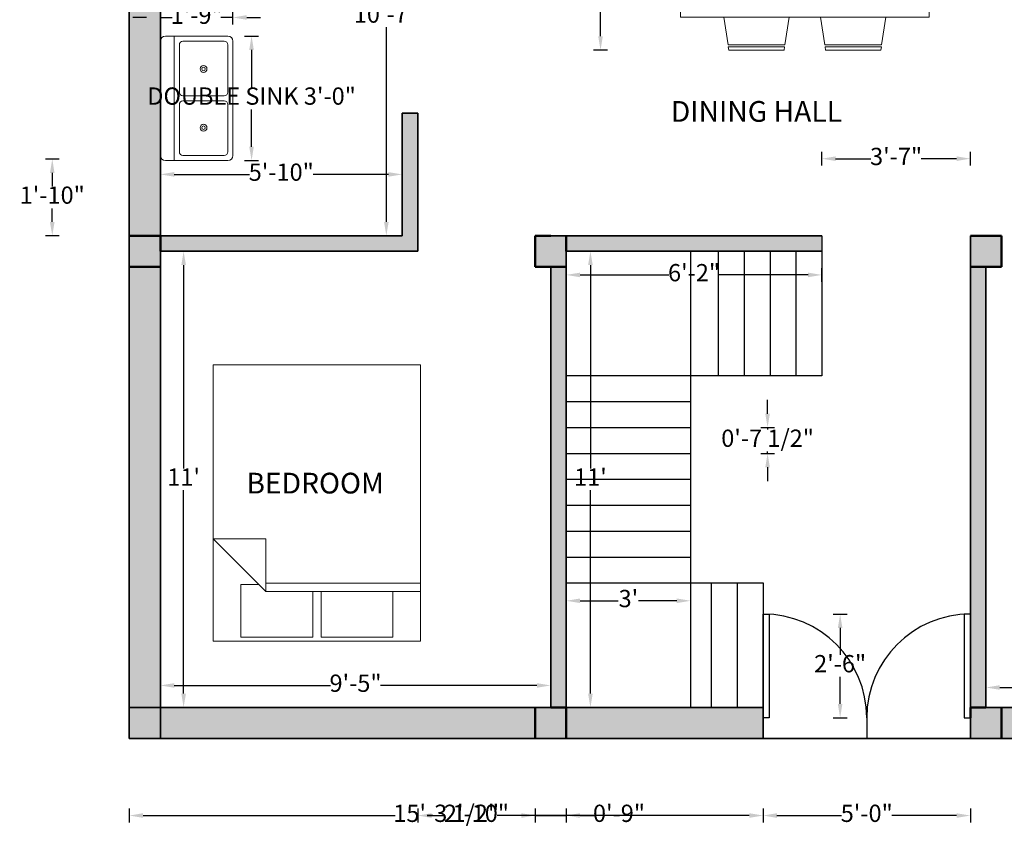
# Model space of a CAD drawing. Units: inches. Extents: x 2244 to 2676, y 593 to 1067.
# Tile 1 of 4: x 2244 to 2530, y 593 to 831. Entities that reach past the tile are written whole.
import ezdxf

# ---------------------------------------------------------------- set-up
doc = ezdxf.new("R2010")
doc.units = ezdxf.units.IN
for name, color, linetype, lineweight in [('A-ANNO-DIMS', 2, 'Continuous', 18), ('A-AREA-IDEN', 7, 'Continuous', 25), ('A-COLS', 7, 'Continuous', 50), ('A-COLS-PATT', 1, 'Continuous', 13), ('A-DOOR', 4, 'Continuous', 25), ('A-FLOR-FIXT', 9, 'Continuous', 18), ('A-FLOR-STRS', 7, 'Continuous', 25), ('A-FURN', 8, 'Continuous', 18), ('A-WALL', 7, 'Continuous', 35)]:
    doc.layers.add(name, color=color, linetype=linetype, lineweight=lineweight)
doc.layers.add('A-WALL-PATT', color=159, linetype='Continuous', lineweight=13, true_color=0x22346e)
doc.styles.get("Standard").update_dxf_attribs({"font": 'arial.ttf'})
doc.dimstyles.new('ISO-25', dxfattribs={"dimtxt": 5, "dimasz": 4, "dimexe": 2, "dimexo": 2, "dimtad": 0, "dimtih": 1, "dimtoh": 1, "dimlunit": 3, "dimtxsty": 'Standard', "dimcen": 2.5, "dimadec": 0, "dimazin": 0, "dimtfac": 1, "dimtmove": 0, "dimatfit": 3, "dimfxl": 2, "dimfxlon": 1, "dimarcsym": 0})

# ---------------------------------------------------------------- blocks, each defined once
blk = doc.blocks.new('*U2')
for p, q in [((0, 0), (0, -6)), ((30, 0), (30, -6))]:
    blk.add_line(p, q)
blk.add_lwpolyline([(0, 0), (0, 30), (1.75, 30), (1.75, 0)], close=True)
blk.add_arc((0, 0), 30, 0, 90)
blk = doc.blocks.new('*U3')
for p, q in [((-30, 0), (-30, -6)), ((0, 0), (0, -6))]:
    blk.add_line(p, q)
blk.add_lwpolyline([(0, 0), (0, 30), (-1.75, 30), (-1.75, 0)], close=True)
blk.add_arc((0, 0), 30, 90, 180)
blk = doc.blocks.new('*D10')
at = {"layer": 'A-ANNO-DIMS', "color": 0, "lineweight": -2, "transparency": 16777216}
for p, q in [((2285.2, 784.43), (2285.2, 788.17)), ((2355.2, 784.43), (2355.2, 788.17)), ((2289.2, 786.17), (2310.98, 786.17)), ((2351.2, 786.17), (2329.41, 786.17))]:
    blk.add_line(p, q, dxfattribs=at)
at = {"layer": 'A-ANNO-DIMS', "color": 0, "transparency": 16777216}
for points in [[(2289.2, 786.84), (2289.2, 785.5), (2285.2, 786.17)], [(2351.2, 786.84), (2351.2, 785.5), (2355.2, 786.17)]]:
    blk.add_solid(points, dxfattribs=at)
at = {"layer": 'Defpoints', "color": 0, "transparency": 16777216}
for p in [(2355.2, 786.17), (2285.2, 782.43), (2355.2, 782.43)]:
    blk.add_point(p, dxfattribs=at)
at = {"layer": 'A-ANNO-DIMS', "color": 0, "transparency": 16777216, "insert": (2320.2, 786.17), "char_height": 5, "attachment_point": 5}
blk.add_mtext('5\'-10"', dxfattribs=at)
blk = doc.blocks.new('*D15')
at = {"layer": 'A-ANNO-DIMS', "color": 0, "lineweight": -2, "transparency": 16777216}
for p, q in [((2524.2, 639.68), (2524.2, 635.68)), ((2637.2, 639.68), (2637.2, 635.68)), ((2528.2, 637.68), (2573.43, 637.68)), ((2633.2, 637.68), (2587.97, 637.68))]:
    blk.add_line(p, q, dxfattribs=at)
at = {"layer": 'A-ANNO-DIMS', "color": 0, "transparency": 16777216}
for points in [[(2528.2, 638.34), (2528.2, 637.01), (2524.2, 637.68)], [(2633.2, 638.34), (2633.2, 637.01), (2637.2, 637.68)]]:
    blk.add_solid(points, dxfattribs=at)
at = {"layer": 'Defpoints', "color": 0, "transparency": 16777216}
for p in [(2524.2, 645.95), (2637.2, 645.95), (2637.2, 637.68)]:
    blk.add_point(p, dxfattribs=at)
at = {"layer": 'A-ANNO-DIMS', "color": 0, "transparency": 16777216, "insert": (2580.7, 637.68), "char_height": 5, "attachment_point": 5}
blk.add_mtext('9\'-5"', dxfattribs=at)
blk = doc.blocks.new('*D16')
at = {"layer": 'A-ANNO-DIMS', "color": 0, "lineweight": -2, "transparency": 16777216}
for p, q in [((2402.7, 755.08), (2402.7, 759.08)), ((2476.7, 755.08), (2476.7, 759.08)), ((2406.7, 757.08), (2432.41, 757.08)), ((2472.7, 757.08), (2446.98, 757.08))]:
    blk.add_line(p, q, dxfattribs=at)
at = {"layer": 'A-ANNO-DIMS', "color": 0, "transparency": 16777216}
for points in [[(2406.7, 757.74), (2406.7, 756.41), (2402.7, 757.08)], [(2472.7, 757.74), (2472.7, 756.41), (2476.7, 757.08)]]:
    blk.add_solid(points, dxfattribs=at)
at = {"layer": 'Defpoints', "color": 0, "transparency": 16777216}
for p in [(2476.7, 757.08), (2402.7, 743.42), (2476.7, 743.42)]:
    blk.add_point(p, dxfattribs=at)
at = {"layer": 'A-ANNO-DIMS', "color": 0, "transparency": 16777216, "insert": (2439.7, 757.08), "char_height": 5, "attachment_point": 5}
blk.add_mtext('6\'-2"', dxfattribs=at)
blk = doc.blocks.new('*D17')
at = {"layer": 'A-ANNO-DIMS', "color": 0, "lineweight": -2, "transparency": 16777216}
for p, q in [((2411.7, 763.92), (2407.7, 763.92)), ((2409.7, 759.92), (2409.7, 701.06)), ((2409.7, 635.92), (2409.7, 694.79)), ((2411.7, 631.92), (2407.7, 631.92))]:
    blk.add_line(p, q, dxfattribs=at)
at = {"layer": 'A-ANNO-DIMS', "color": 0, "transparency": 16777216}
for points in [[(2409.03, 759.92), (2410.37, 759.92), (2409.7, 763.92)], [(2409.03, 635.92), (2410.37, 635.92), (2409.7, 631.92)]]:
    blk.add_solid(points, dxfattribs=at)
at = {"layer": 'Defpoints', "color": 0, "transparency": 16777216}
for p in [(2415.93, 763.92), (2409.7, 631.92), (2415.93, 631.92)]:
    blk.add_point(p, dxfattribs=at)
at = {"layer": 'A-ANNO-DIMS', "color": 0, "transparency": 16777216, "insert": (2409.7, 697.92), "char_height": 5, "attachment_point": 5}
blk.add_mtext("11'", dxfattribs=at)
blk = doc.blocks.new('*D18')
at = {"layer": 'A-ANNO-DIMS', "color": 0, "lineweight": -2, "transparency": 16777216}
for p, q in [((2402.7, 664.77), (2402.7, 660.77)), ((2438.7, 664.77), (2438.7, 660.77)), ((2406.7, 662.77), (2417.77, 662.77)), ((2434.7, 662.77), (2423.62, 662.77))]:
    blk.add_line(p, q, dxfattribs=at)
at = {"layer": 'A-ANNO-DIMS', "color": 0, "transparency": 16777216}
for points in [[(2406.7, 663.44), (2406.7, 662.11), (2402.7, 662.77)], [(2434.7, 663.44), (2434.7, 662.11), (2438.7, 662.77)]]:
    blk.add_solid(points, dxfattribs=at)
at = {"layer": 'Defpoints', "color": 0, "transparency": 16777216}
for p in [(2402.7, 667.92), (2438.7, 667.92), (2438.7, 662.77)]:
    blk.add_point(p, dxfattribs=at)
at = {"layer": 'A-ANNO-DIMS', "color": 0, "transparency": 16777216, "insert": (2420.7, 662.77), "char_height": 5, "attachment_point": 5}
blk.add_mtext("3'", dxfattribs=at)
blk = doc.blocks.new('*D19')
at = {"layer": 'A-ANNO-DIMS', "color": 0, "lineweight": -2, "transparency": 16777216}
for p, q in [((2291.93, 763.92), (2289.93, 763.92)), ((2291.93, 759.92), (2291.93, 701.06)), ((2291.93, 635.92), (2291.93, 694.79)), ((2291.93, 631.92), (2289.93, 631.92))]:
    blk.add_line(p, q, dxfattribs=at)
at = {"layer": 'A-ANNO-DIMS', "color": 0, "transparency": 16777216}
for points in [[(2291.27, 759.92), (2292.6, 759.92), (2291.93, 763.92)], [(2291.27, 635.92), (2292.6, 635.92), (2291.93, 631.92)]]:
    blk.add_solid(points, dxfattribs=at)
at = {"layer": 'Defpoints', "color": 0, "transparency": 16777216}
for p in [(2292.44, 763.92), (2291.93, 631.92), (2292.44, 631.92)]:
    blk.add_point(p, dxfattribs=at)
at = {"layer": 'A-ANNO-DIMS', "color": 0, "transparency": 16777216, "insert": (2291.93, 697.92), "char_height": 5, "attachment_point": 5}
blk.add_mtext("11'", dxfattribs=at)
blk = doc.blocks.new('*D20')
at = {"layer": 'A-ANNO-DIMS', "color": 0, "lineweight": -2, "transparency": 16777216}
for p, q in [((2285.2, 640.27), (2285.2, 636.27)), ((2398.2, 640.27), (2398.2, 636.27)), ((2289.2, 638.27), (2334.43, 638.27)), ((2394.2, 638.27), (2348.97, 638.27))]:
    blk.add_line(p, q, dxfattribs=at)
at = {"layer": 'A-ANNO-DIMS', "color": 0, "transparency": 16777216}
for points in [[(2289.2, 638.93), (2289.2, 637.6), (2285.2, 638.27)], [(2394.2, 638.93), (2394.2, 637.6), (2398.2, 638.27)]]:
    blk.add_solid(points, dxfattribs=at)
at = {"layer": 'Defpoints', "color": 0, "transparency": 16777216}
for p in [(2285.2, 662.54), (2398.2, 662.54), (2398.2, 638.27)]:
    blk.add_point(p, dxfattribs=at)
at = {"layer": 'A-ANNO-DIMS', "color": 0, "transparency": 16777216, "insert": (2341.7, 638.27), "char_height": 5, "attachment_point": 5}
blk.add_mtext('9\'-5"', dxfattribs=at)
blk = doc.blocks.new('Bed - Queen')
for p, q in [((0, -80.00003), (0, 0)), ((0, 0), (59.99999, 0)), ((59.99999, 0), (59.99999, -80.00003)), ((7.99999, -1.2), (28.79998, -1.2)), ((7.99999, -14.4), (7.99999, -1.2)), ((28.79998, -1.2), (28.79998, -14.4)), ((31.19999, -1.2), (51.99999, -1.2)), ((31.19999, -14.4), (31.19999, -1.2)), ((51.99999, -1.2), (51.99999, -16.4)), ((0, -14.4), (44.8, -14.4)), ((44.8, -16.8), (0, -16.8)), ((59.99999, -29.6), (44.8, -14.4)), ((44.8, -14.4), (44.8, -29.6)), ((51.99999, -16.4), (46.79936, -16.4)), ((44.8, -29.6), (59.99999, -29.6)), ((59.99999, -80.00003), (0, -80.00003))]:
    blk.add_line(p, q)
blk = doc.blocks.new('Dining Set - 36 x 72 in.')
for p, q in [((-22.2343, 26.00059), (-23.4847, 17.99762)), ((-22.2304, 26), (-5.7608, 26)), ((-22, 27.5), (-22.1562, 26.50042)), ((-5.8416, 26.5), (-22.1534, 26.5)), ((-22, 27.5), (-6, 27.5)), ((-5.8437, 26.49966), (-6, 27.5)), ((-4.5152, 17.99762), (-5.7655, 25.99926)), ((5.7657, 26.00059), (4.5153, 17.99762)), ((5.7696, 26), (22.2392, 26)), ((6, 27.5), (5.8438, 26.50042)), ((22.1584, 26.5), (5.8466, 26.5)), ((6, 27.5), (22, 27.5)), ((22.1563, 26.49966), (22, 27.5)), ((23.4848, 17.99762), (22.2345, 25.99926)), ((36, 18), (-36, 18)), ((-36, 18), (-36, -18)), ((36, -18), (36, 18)), ((-44.0006, 8.23428), (-35.9976, 9.48474)), ((44.0006, 8.23428), (35.9976, 9.48474)), ((-45.5, 8), (-44.5004, 8.15617)), ((-45.5, 8), (-45.5, -8)), ((-44.5, -8.15843), (-44.5, 8.15338)), ((-44, 8.23041), (-44, -8.23915)), ((44, 8.23041), (44, -8.23915)), ((44.5, -8.15843), (44.5, 8.15338)), ((45.5, 8), (44.5005, 8.15617)), ((45.5, 8), (45.5, -8)), ((-44.4997, -8.15631), (-45.5, -8)), ((-35.9976, -9.48476), (-43.9993, -8.2345)), ((35.9976, -9.48476), (43.9993, -8.2345)), ((44.4997, -8.15631), (45.5, -8)), ((-36, -18), (36, -18)), ((-22.2343, -26.0006), (-23.4847, -17.99762)), ((-4.5152, -17.99762), (-5.7655, -25.99928)), ((5.7657, -26.0006), (4.5153, -17.99762)), ((23.4848, -17.99762), (22.2345, -25.99928)), ((-22.2304, -26), (-5.7608, -26)), ((-22, -27.5), (-22.1562, -26.50044)), ((-5.8416, -26.5), (-22.1534, -26.5)), ((-22, -27.5), (-6, -27.5)), ((-5.8437, -26.49967), (-6, -27.5)), ((5.7696, -26), (22.2392, -26)), ((6, -27.5), (5.8438, -26.50044)), ((22.1584, -26.5), (5.8466, -26.5)), ((6, -27.5), (22, -27.5)), ((22.1563, -26.49967), (22, -27.5))]:
    blk.add_line(p, q)
for points in [[(-36, 15), (-31.1772, 14.97754), (-26.8079, 14.91406), (-22.8538, 14.81543), (-19.276, 14.6875), (-16.0362, 14.53613), (-13.0957, 14.36718), (-10.4159, 14.18652), (-7.9583, 14), (-5.6904, 13.81315), (-3.6035, 13.63021), (-1.6954, 13.45508), (0.0365, 13.29166), (1.5945, 13.14388), (2.9811, 13.01562), (4.1988, 12.9108), (5.25, 12.83333), (6.1393, 12.78613), (6.8802, 12.76823), (7.4883, 12.77767), (7.9792, 12.8125), (8.3685, 12.87077), (8.6719, 12.95052), (8.9049, 13.0498), (9.0833, 13.16666), (9.2205, 13.29899), (9.3216, 13.44401), (9.3895, 13.59879), (9.4271, 13.76041), (9.4373, 13.92594), (9.4232, 14.09245), (9.3875, 14.257), (9.3333, 14.41666), (9.2638, 14.56917), (9.1836, 14.71484), (9.0975, 14.85465), (9.0104, 14.98958), (8.9272, 15.1206), (8.8529, 15.2487), (8.7922, 15.37483), (8.75, 15.5), (8.7305, 15.62467), (8.7344, 15.74739), (8.7617, 15.86621), (8.8125, 15.97916), (8.8867, 16.08431), (8.9844, 16.17968), (9.1055, 16.26334), (9.25, 16.33333), (9.4189, 16.38802), (9.6172, 16.42708), (9.8506, 16.45052), (10.125, 16.45833), (10.4463, 16.45052), (10.8203, 16.42708), (11.2529, 16.38802), (11.75, 16.33333), (12.3184, 16.26318), (12.9694, 16.17838), (13.7151, 16.07991), (14.5677, 15.96875), (15.5395, 15.84586), (16.6426, 15.71224), (17.8893, 15.56884), (19.2917, 15.41666), (20.859, 15.25667), (22.5879, 15.08984), (24.4721, 14.91715), (26.5052, 14.73958), (28.6809, 14.5581), (30.9929, 14.3737), (33.4347, 14.18733), (36, 14)], [(-36, 10), (-28.9766, 10.14274), (-23.1725, 10.20442), (-18.4241, 10.19775), (-14.5677, 10.13541), (-11.4399, 10.03011), (-8.877, 9.89453), (-6.7154, 9.74137), (-4.7917, 9.58333), (-2.9698, 9.43082), (-1.2246, 9.28515), (0.4415, 9.14534), (2.026, 9.01041), (3.5266, 8.87939), (4.9408, 8.7513), (6.266, 8.62516), (7.5, 8.5), (8.6411, 8.37549), (9.6914, 8.2539), (10.6538, 8.13818), (11.5312, 8.03125), (12.3267, 7.93603), (13.043, 7.85547), (13.6831, 7.79248), (14.25, 7.75), (14.7471, 7.7303), (15.1797, 7.73307), (15.5537, 7.75732), (15.875, 7.80208), (16.1494, 7.86637), (16.3828, 7.94922), (16.5811, 8.04964), (16.75, 8.16666), (16.8944, 8.29915), (17.0143, 8.44531), (17.1089, 8.60319), (17.1771, 8.77083), (17.218, 8.94629), (17.2305, 9.1276), (17.2137, 9.31282), (17.1667, 9.5), (17.0895, 9.6875), (16.987, 9.875), (16.8649, 10.0625), (16.7292, 10.25), (16.5856, 10.4375), (16.4401, 10.625), (16.2985, 10.8125), (16.1667, 11), (16.05, 11.18733), (15.9518, 11.3737), (15.8752, 11.5581), (15.8229, 11.73958), (15.798, 11.91715), (15.8034, 12.08984), (15.842, 12.25667), (15.9167, 12.41666), (16.0295, 12.56836), (16.1784, 12.70833), (16.3605, 12.83268), (16.5729, 12.9375), (16.8127, 13.01888), (17.0768, 13.07291), (17.3625, 13.0957), (17.6667, 13.08333), (17.9894, 13.03312), (18.3418, 12.94726), (18.7382, 12.82918), (19.1927, 12.68229), (19.7195, 12.51001), (20.3327, 12.31575), (21.0465, 12.10294), (21.875, 11.875), (22.8357, 11.63354), (23.959, 11.37304), (25.2786, 11.08618), (26.8282, 10.76562), (28.6414, 10.40405), (30.752, 9.99414), (33.1936, 9.52856), (36, 9)], [(-36, 5.5), (-30.7157, 5.3348), (-26.069, 5.20963), (-21.9946, 5.11767), (-18.4271, 5.05208), (-15.3009, 5.00602), (-12.5508, 4.97265), (-10.1112, 4.94515), (-7.9167, 4.91666), (-5.909, 4.88167), (-4.0586, 4.83984), (-2.3429, 4.79215), (-0.7396, 4.73958), (0.7739, 4.6831), (2.22, 4.6237), (3.6213, 4.56233), (5, 4.5), (6.373, 4.43782), (7.7344, 4.3776), (9.0723, 4.32129), (10.375, 4.27083), (11.6309, 4.22819), (12.8281, 4.19531), (13.9551, 4.17415), (15, 4.16666), (15.954, 4.17448), (16.819, 4.19791), (17.6001, 4.23698), (18.3021, 4.29166), (18.9299, 4.36198), (19.4883, 4.44791), (19.9823, 4.54948), (20.4167, 4.66666), (20.7969, 4.79899), (21.1302, 4.94401), (21.4245, 5.09879), (21.6875, 5.26041), (21.9271, 5.42594), (22.1511, 5.59245), (22.3672, 5.757), (22.5834, 5.91666), (22.8065, 6.06868), (23.0404, 6.21093), (23.2879, 6.34147), (23.5521, 6.45833), (23.8358, 6.55957), (24.142, 6.64323), (24.4735, 6.70735), (24.8334, 6.75), (25.2235, 6.76969), (25.642, 6.76692), (26.0858, 6.74267), (26.5521, 6.69791), (27.0379, 6.63362), (27.5404, 6.55078), (28.0565, 6.45036), (28.5834, 6.33333), (29.1242, 6.19987), (29.7071, 6.04687), (30.3661, 5.87044), (31.1354, 5.66666), (32.0493, 5.43164), (33.142, 5.16146), (34.4475, 4.85221), (36, 4.5)], [(-36, -1), (-30.7915, -0.6591), (-26.0195, -0.38216), (-21.6519, -0.16284), (-17.6563, 0.00521), (-14.0005, 0.12833), (-10.6523, 0.21289), (-7.5796, 0.26522), (-4.75, 0.29166), (-2.134, 0.29793), (0.2878, 0.28711), (2.5317, 0.26163), (4.6146, 0.22396), (6.5529, 0.17651), (8.3633, 0.12174), (10.0623, 0.06209), (11.6667, 0), (13.1899, -0.06201), (14.6341, -0.1211), (15.9982, -0.17432), (17.2813, -0.21875), (18.4823, -0.25147), (19.6003, -0.26953), (20.6343, -0.27002), (21.5834, -0.25), (22.4481, -0.20768), (23.2357, -0.14584), (23.9549, -0.06836), (24.6146, 0.02083), (25.2235, 0.11784), (25.7904, 0.21875), (26.3241, 0.31966), (26.8334, 0.41666), (27.3265, 0.50618), (27.8099, 0.58593), (28.2894, 0.65397), (28.7709, 0.70833), (29.2601, 0.74707), (29.763, 0.76823), (30.2855, 0.76985), (30.8334, 0.75), (31.4088, 0.70784), (31.9994, 0.64713), (32.589, 0.57275), (33.1615, 0.48958), (33.7008, 0.4025), (34.1908, 0.3164), (34.6153, 0.23616), (34.9584, 0.16666), (35.2099, 0.11165), (35.3848, 0.07031), (35.504, 0.04069), (35.5886, 0.02083), (35.6594, 0.00879), (35.7377, 0.0026), (35.8442, 0.00032), (36, 0)], [(-36, -6.5), (-27.1843, -6.31267), (-20.084, -6.1263), (-14.469, -5.9419), (-10.1094, -5.76042), (-6.7752, -5.58285), (-4.2363, -5.41016), (-2.2629, -5.24333), (-0.625, -5.08334), (0.8708, -4.93099), (2.2715, -4.78646), (3.5872, -4.64974), (4.8281, -4.52084), (6.0046, -4.39974), (7.127, -4.28646), (8.2053, -4.18099), (9.25, -4.08334), (10.2705, -3.99382), (11.2734, -3.91407), (12.2647, -3.84603), (13.25, -3.79167), (14.2354, -3.75293), (15.2266, -3.73177), (16.2295, -3.73015), (17.25, -3.75), (18.2912, -3.79248), (19.3451, -3.85547), (20.4009, -3.93604), (21.4479, -4.03125), (22.4754, -4.13819), (23.4727, -4.25391), (24.4289, -4.37549), (25.3334, -4.5), (26.1785, -4.62492), (26.9694, -4.74935), (27.7145, -4.87281), (28.4219, -4.99479), (29.1, -5.11483), (29.7572, -5.23242), (30.4016, -5.34709), (31.0417, -5.45834), (31.6837, -5.56437), (32.3262, -5.65821), (32.9658, -5.73153), (33.599, -5.77604), (34.2224, -5.78345), (34.8327, -5.74545), (35.4264, -5.65373), (36, -5.5)], [(-36, -10), (-26.4022, -9.81299), (-18.4675, -9.62891), (-11.9839, -9.45069), (-6.7396, -9.28125), (-2.5226, -9.12354), (0.8789, -8.98047), (3.6769, -8.85498), (6.0833, -8.75), (8.2767, -8.66765), (10.3021, -8.60677), (12.1712, -8.56543), (13.8958, -8.54167), (15.4876, -8.53353), (16.9583, -8.53907), (18.3197, -8.55632), (19.5834, -8.58334), (20.7616, -8.61841), (21.8685, -8.66081), (22.9188, -8.71004), (23.9271, -8.76563), (24.9081, -8.82707), (25.8763, -8.89388), (26.8465, -8.96558), (27.8334, -9.04167), (28.8474, -9.12118), (29.8828, -9.20117), (30.93, -9.27824), (31.9792, -9.34896), (33.0205, -9.40991), (34.0443, -9.45768), (35.0407, -9.48885), (36, -9.5)], [(-36, -14.5), (-30.0881, -14.33513), (-25.0332, -14.21224), (-20.7312, -14.12647), (-17.0781, -14.07292), (-13.97, -14.04671), (-11.3027, -14.04297), (-8.9724, -14.05681), (-6.875, -14.08334), (-4.9224, -14.11833), (-3.0905, -14.16016), (-1.3709, -14.20785), (0.2448, -14.26042), (1.7647, -14.3169), (3.1973, -14.3763), (4.5507, -14.43767), (5.8333, -14.5), (7.0554, -14.5621), (8.235, -14.62175), (9.3922, -14.67652), (10.5469, -14.72396), (11.7192, -14.76164), (12.929, -14.78711), (14.1965, -14.79794), (15.5417, -14.79167), (16.9933, -14.76424), (18.6152, -14.70508), (20.4804, -14.60197), (22.6615, -14.44271), (25.2312, -14.21509), (28.2624, -13.9069), (31.8277, -13.50594), (36, -13)]]:
    blk.add_lwpolyline(points)
blk = doc.blocks.new('Sink-double - 36 in top')
for p, q in [((-18, -4), (18, -4)), ((-0.75, -18.5), (-0.75, -6.5)), ((0.75, -6.5), (0.75, -18.5))]:
    blk.add_line(p, q)
for points in [[(-16.5, 0), (16.5, 0)], [(-18, -19.5), (-18, -1.5)], [(18, -1.5), (18, -19.5)], [(-15.5, -5.5), (-1.75, -5.5)], [(1.75, -5.5), (15.5, -5.5)], [(-16.5, -18.5), (-16.5, -6.5)], [(16.5, -6.5), (16.5, -18.5)], [(-1.75, -19.5), (-15.5, -19.5)], [(15.5, -19.5), (1.75, -19.5)], [(16.5, -21), (-16.5, -21)]]:
    blk.add_lwpolyline(points)
for centre, radius in [((-8.5, -12.5), 1), ((-8.5, -12.5), 0.5), ((8.5, -12.5), 1), ((8.5, -12.5), 0.5)]:
    blk.add_circle(centre, radius)
for centre, radius, start, end in [((-16.5, -1.5), 1.5, 90, 180), ((16.5, -1.5), 1.5, 0, 90), ((-15.5, -6.5), 1, 90, 180), ((-1.75, -6.5), 1, 0, 90), ((1.75, -6.5), 1, 90, 180), ((15.5, -6.5), 1, 0, 90), ((-16.5, -19.5), 1.5, 180, 270), ((-15.5, -18.5), 1, 180, 270), ((-1.75, -18.5), 1, 270, 0), ((1.75, -18.5), 1, 180, 270), ((15.5, -18.5), 1, 270, 0), ((16.5, -19.5), 1.5, 270, 0)]:
    blk.add_arc(centre, radius, start, end)
blk = doc.blocks.new('*D28')
at = {"layer": 'A-ANNO-DIMS', "color": 0, "lineweight": -2, "transparency": 16777216}
for p, q in [((2352.62, 895.42), (2348.62, 895.42)), ((2350.62, 891.42), (2350.62, 835.1)), ((2350.62, 772.42), (2350.62, 828.74)), ((2352.62, 768.42), (2348.62, 768.42))]:
    blk.add_line(p, q, dxfattribs=at)
at = {"layer": 'A-ANNO-DIMS', "color": 0, "transparency": 16777216}
for points in [[(2349.96, 891.42), (2351.29, 891.42), (2350.62, 895.42)], [(2349.96, 772.42), (2351.29, 772.42), (2350.62, 768.42)]]:
    blk.add_solid(points, dxfattribs=at)
at = {"layer": 'Defpoints', "color": 0, "transparency": 16777216}
for p in [(2355.2, 895.42), (2350.62, 768.42), (2355.2, 768.42)]:
    blk.add_point(p, dxfattribs=at)
at = {"layer": 'A-ANNO-DIMS', "color": 0, "transparency": 16777216, "insert": (2350.62, 831.92), "char_height": 5, "attachment_point": 5}
blk.add_mtext('10\'-7"', dxfattribs=at)
blk = doc.blocks.new('*D33')
at = {"layer": 'A-ANNO-DIMS', "color": 0, "lineweight": -2, "transparency": 16777216}
for p, q in [((2414.63, 877.13), (2410.63, 877.13)), ((2412.63, 873.13), (2412.63, 852.75)), ((2412.63, 826.13), (2412.63, 846.5)), ((2414.63, 822.13), (2410.63, 822.13))]:
    blk.add_line(p, q, dxfattribs=at)
at = {"layer": 'A-ANNO-DIMS', "color": 0, "transparency": 16777216}
for points in [[(2411.96, 873.13), (2413.3, 873.13), (2412.63, 877.13)], [(2411.96, 826.13), (2413.3, 826.13), (2412.63, 822.13)]]:
    blk.add_solid(points, dxfattribs=at)
at = {"layer": 'Defpoints', "color": 0, "transparency": 16777216}
for p in [(2412.63, 877.13), (2426.28, 877.13), (2426.28, 822.13)]:
    blk.add_point(p, dxfattribs=at)
at = {"layer": 'A-ANNO-DIMS', "color": 0, "transparency": 16777216, "insert": (2412.63, 849.63), "char_height": 5, "attachment_point": 5}
blk.add_mtext('4\'-7"', dxfattribs=at)
blk = doc.blocks.new('*D36')
at = {"layer": 'A-ANNO-DIMS', "color": 0, "lineweight": -2, "transparency": 16777216}
for p, q in [((2309.6, 826.19), (2313.6, 826.19)), ((2311.6, 822.19), (2311.6, 811.4)), ((2311.6, 794.19), (2311.6, 804.97)), ((2309.6, 790.19), (2313.6, 790.19))]:
    blk.add_line(p, q, dxfattribs=at)
at = {"layer": 'A-ANNO-DIMS', "color": 0, "transparency": 16777216}
for points in [[(2310.93, 822.19), (2312.26, 822.19), (2311.6, 826.19)], [(2310.93, 794.19), (2312.26, 794.19), (2311.6, 790.19)]]:
    blk.add_solid(points, dxfattribs=at)
at = {"layer": 'Defpoints', "color": 0, "transparency": 16777216}
for p in [(2306.2, 826.19), (2311.6, 826.19), (2306.2, 790.19)]:
    blk.add_point(p, dxfattribs=at)
at = {"layer": 'A-ANNO-DIMS', "color": 0, "transparency": 16777216, "insert": (2311.6, 808.19), "char_height": 5, "attachment_point": 5}
blk.add_mtext('DOUBLE SINK 3\'-0"', dxfattribs=at)
blk = doc.blocks.new('*D37')
at = {"layer": 'A-ANNO-DIMS', "color": 0, "lineweight": -2, "transparency": 16777216}
for p, q in [((2285.2, 829.59), (2285.2, 833.59)), ((2306.2, 829.59), (2306.2, 833.59)), ((2281.2, 831.59), (2277.2, 831.59)), ((2285.2, 831.59), (2288.66, 831.59)), ((2306.2, 831.59), (2302.73, 831.59)), ((2310.2, 831.59), (2314.2, 831.59))]:
    blk.add_line(p, q, dxfattribs=at)
at = {"layer": 'A-ANNO-DIMS', "color": 0, "transparency": 16777216}
for points in [[(2281.2, 832.25), (2281.2, 830.92), (2285.2, 831.59)], [(2310.2, 832.25), (2310.2, 830.92), (2306.2, 831.59)]]:
    blk.add_solid(points, dxfattribs=at)
at = {"layer": 'Defpoints', "color": 0, "transparency": 16777216}
for p in [(2285.2, 831.59), (2285.2, 826.19), (2306.2, 826.19)]:
    blk.add_point(p, dxfattribs=at)
at = {"layer": 'A-ANNO-DIMS', "color": 0, "transparency": 16777216, "insert": (2295.7, 831.59), "char_height": 5, "attachment_point": 5}
blk.add_mtext('1\'-9"', dxfattribs=at)
blk = doc.blocks.new('*D40')
at = {"layer": 'A-ANNO-DIMS', "color": 0, "lineweight": -2, "transparency": 16777216}
for p, q in [((2276.2, 602.62), (2276.2, 598.62)), ((2459.7, 602.62), (2459.7, 598.62)), ((2280.2, 600.62), (2353.14, 600.62)), ((2455.7, 600.62), (2382.75, 600.62))]:
    blk.add_line(p, q, dxfattribs=at)
at = {"layer": 'A-ANNO-DIMS', "color": 0, "transparency": 16777216}
for points in [[(2280.2, 601.29), (2280.2, 599.95), (2276.2, 600.62)], [(2455.7, 601.29), (2455.7, 599.95), (2459.7, 600.62)]]:
    blk.add_solid(points, dxfattribs=at)
at = {"layer": 'Defpoints', "color": 0, "transparency": 16777216}
for p in [(2276.2, 622.92), (2459.7, 622.92), (2459.7, 600.62)]:
    blk.add_point(p, dxfattribs=at)
at = {"layer": 'A-ANNO-DIMS', "color": 0, "transparency": 16777216, "insert": (2367.95, 600.62), "char_height": 5, "attachment_point": 5}
blk.add_mtext('15\'-3 1/2"', dxfattribs=at)
blk = doc.blocks.new('*D41')
at = {"layer": 'A-ANNO-DIMS', "color": 0, "lineweight": -2, "transparency": 16777216}
for p, q in [((2459.7, 602.62), (2459.7, 598.62)), ((2519.7, 602.62), (2519.7, 598.62)), ((2463.7, 600.62), (2482.43, 600.62)), ((2515.7, 600.62), (2496.97, 600.62))]:
    blk.add_line(p, q, dxfattribs=at)
at = {"layer": 'A-ANNO-DIMS', "color": 0, "transparency": 16777216}
for points in [[(2463.7, 601.29), (2463.7, 599.95), (2459.7, 600.62)], [(2515.7, 601.29), (2515.7, 599.95), (2519.7, 600.62)]]:
    blk.add_solid(points, dxfattribs=at)
at = {"layer": 'Defpoints', "color": 0, "transparency": 16777216}
for p in [(2459.7, 622.92), (2519.7, 622.92), (2519.7, 600.62)]:
    blk.add_point(p, dxfattribs=at)
at = {"layer": 'A-ANNO-DIMS', "color": 0, "transparency": 16777216, "insert": (2489.7, 600.62), "char_height": 5, "attachment_point": 5}
blk.add_mtext('5\'-0"', dxfattribs=at)
blk = doc.blocks.new('*D42')
at = {"layer": 'A-ANNO-DIMS', "color": 0, "lineweight": -2, "transparency": 16777216}
for p, q in [((2666.5, 859.92), (2670.5, 859.92)), ((2668.5, 855.92), (2668.5, 835.1)), ((2668.5, 807.92), (2668.5, 828.74)), ((2666.5, 803.92), (2670.5, 803.92))]:
    blk.add_line(p, q, dxfattribs=at)
at = {"layer": 'A-ANNO-DIMS', "color": 0, "transparency": 16777216}
for points in [[(2667.83, 855.92), (2669.16, 855.92), (2668.5, 859.92)], [(2667.83, 807.92), (2669.16, 807.92), (2668.5, 803.92)]]:
    blk.add_solid(points, dxfattribs=at)
at = {"layer": 'Defpoints', "color": 0, "transparency": 16777216}
for p in [(2359.7, 859.92), (2668.5, 859.92), (2359.7, 803.92)]:
    blk.add_point(p, dxfattribs=at)
at = {"layer": 'A-ANNO-DIMS', "color": 0, "transparency": 16777216, "insert": (2668.5, 831.92), "char_height": 5, "attachment_point": 5}
blk.add_mtext('4\'-8"', dxfattribs=at)
blk = doc.blocks.new('*D43')
at = {"layer": 'A-ANNO-DIMS', "color": 0, "lineweight": -2, "transparency": 16777216}
for p, q in [((2359.7, 602.62), (2359.7, 598.62)), ((2393.7, 602.62), (2393.7, 598.62)), ((2363.7, 600.62), (2367.44, 600.62)), ((2389.7, 600.62), (2385.95, 600.62))]:
    blk.add_line(p, q, dxfattribs=at)
at = {"layer": 'A-ANNO-DIMS', "color": 0, "transparency": 16777216}
for points in [[(2363.7, 601.29), (2363.7, 599.95), (2359.7, 600.62)], [(2389.7, 601.29), (2389.7, 599.95), (2393.7, 600.62)]]:
    blk.add_solid(points, dxfattribs=at)
at = {"layer": 'Defpoints', "color": 0, "transparency": 16777216}
for p in [(2393.7, 768.42), (2359.7, 763.92), (2393.7, 600.62)]:
    blk.add_point(p, dxfattribs=at)
at = {"layer": 'A-ANNO-DIMS', "color": 0, "transparency": 16777216, "insert": (2376.7, 600.62), "char_height": 5, "attachment_point": 5}
blk.add_mtext('2\'-10"', dxfattribs=at)
blk = doc.blocks.new('*D50')
at = {"layer": 'A-ANNO-DIMS', "color": 0, "lineweight": -2, "transparency": 16777216}
for p, q in [((2476.7, 788.72), (2476.7, 792.72)), ((2519.7, 788.72), (2519.7, 792.72)), ((2480.7, 790.72), (2490.93, 790.72)), ((2515.7, 790.72), (2505.47, 790.72))]:
    blk.add_line(p, q, dxfattribs=at)
at = {"layer": 'A-ANNO-DIMS', "color": 0, "transparency": 16777216}
for points in [[(2480.7, 791.39), (2480.7, 790.05), (2476.7, 790.72)], [(2515.7, 791.39), (2515.7, 790.05), (2519.7, 790.72)]]:
    blk.add_solid(points, dxfattribs=at)
at = {"layer": 'Defpoints', "color": 0, "transparency": 16777216}
for p in [(2519.7, 790.72), (2476.7, 768.42), (2519.7, 768.42)]:
    blk.add_point(p, dxfattribs=at)
at = {"layer": 'A-ANNO-DIMS', "color": 0, "transparency": 16777216, "insert": (2498.2, 790.72), "char_height": 5, "attachment_point": 5}
blk.add_mtext('3\'-7"', dxfattribs=at)
blk = doc.blocks.new('*D52')
at = {"layer": 'A-ANNO-DIMS', "color": 0, "lineweight": -2, "transparency": 16777216}
for p, q in [((2255.9, 790.62), (2251.9, 790.62)), ((2253.9, 786.62), (2253.9, 782.7)), ((2253.9, 772.42), (2253.9, 776.35)), ((2255.9, 768.42), (2251.9, 768.42))]:
    blk.add_line(p, q, dxfattribs=at)
at = {"layer": 'A-ANNO-DIMS', "color": 0, "transparency": 16777216}
for points in [[(2253.23, 786.62), (2254.56, 786.62), (2253.9, 790.62)], [(2253.23, 772.42), (2254.56, 772.42), (2253.9, 768.42)]]:
    blk.add_solid(points, dxfattribs=at)
at = {"layer": 'Defpoints', "color": 0, "transparency": 16777216}
for p in [(2253.9, 790.62), (2285.64, 790.62), (2285.2, 768.42)]:
    blk.add_point(p, dxfattribs=at)
at = {"layer": 'A-ANNO-DIMS', "color": 0, "transparency": 16777216, "insert": (2253.9, 779.52), "char_height": 5, "attachment_point": 5}
blk.add_mtext('1\'-10"', dxfattribs=at)
blk = doc.blocks.new('*D55')
at = {"layer": 'A-ANNO-DIMS', "color": 0, "lineweight": -2, "transparency": 16777216}
for p, q in [((2461, 716.92), (2461, 720.92)), ((2459, 712.92), (2463, 712.92)), ((2461, 712.92), (2461, 712.38)), ((2459, 705.42), (2463, 705.42)), ((2461, 705.42), (2461, 705.96)), ((2461, 701.42), (2461, 697.42))]:
    blk.add_line(p, q, dxfattribs=at)
at = {"layer": 'A-ANNO-DIMS', "color": 0, "transparency": 16777216}
for points in [[(2460.33, 716.92), (2461.66, 716.92), (2461, 712.92)], [(2460.33, 701.42), (2461.66, 701.42), (2461, 705.42)]]:
    blk.add_solid(points, dxfattribs=at)
at = {"layer": 'Defpoints', "color": 0, "transparency": 16777216}
for p in [(2438.7, 712.92), (2438.7, 705.42), (2461, 705.42)]:
    blk.add_point(p, dxfattribs=at)
at = {"layer": 'A-ANNO-DIMS', "color": 0, "transparency": 16777216, "insert": (2461, 709.17), "char_height": 5, "attachment_point": 5}
blk.add_mtext('0\'-7 1/2"', dxfattribs=at)
blk = doc.blocks.new('*D56')
at = {"layer": 'A-ANNO-DIMS', "color": 0, "lineweight": -2, "transparency": 16777216}
for p, q in [((2480, 658.92), (2484, 658.92)), ((2482, 654.92), (2482, 647.1)), ((2482, 632.92), (2482, 640.74)), ((2480, 628.92), (2484, 628.92))]:
    blk.add_line(p, q, dxfattribs=at)
at = {"layer": 'A-ANNO-DIMS', "color": 0, "transparency": 16777216}
for points in [[(2481.33, 654.92), (2482.66, 654.92), (2482, 658.92)], [(2481.33, 632.92), (2482.66, 632.92), (2482, 628.92)]]:
    blk.add_solid(points, dxfattribs=at)
at = {"layer": 'Defpoints', "color": 0, "transparency": 16777216}
for p in [(2459.7, 658.92), (2459.7, 628.92), (2482, 628.92)]:
    blk.add_point(p, dxfattribs=at)
at = {"layer": 'A-ANNO-DIMS', "color": 0, "transparency": 16777216, "insert": (2482, 643.92), "char_height": 5, "attachment_point": 5}
blk.add_mtext('2\'-6"', dxfattribs=at)
blk = doc.blocks.new('*D57')
at = {"layer": 'A-ANNO-DIMS', "color": 0, "lineweight": -2, "transparency": 16777216}
for p, q in [((2393.7, 602.62), (2393.7, 598.62)), ((2402.7, 602.62), (2402.7, 598.62)), ((2389.7, 600.62), (2385.7, 600.62)), ((2393.7, 600.62), (2402.7, 600.62)), ((2406.7, 600.62), (2410.7, 600.62))]:
    blk.add_line(p, q, dxfattribs=at)
at = {"layer": 'A-ANNO-DIMS', "color": 0, "transparency": 16777216}
for points in [[(2389.7, 601.29), (2389.7, 599.95), (2393.7, 600.62)], [(2406.7, 601.29), (2406.7, 599.95), (2402.7, 600.62)]]:
    blk.add_solid(points, dxfattribs=at)
at = {"layer": 'Defpoints', "color": 0, "transparency": 16777216}
for p in [(2393.7, 768.42), (2402.7, 768.42), (2402.7, 600.62)]:
    blk.add_point(p, dxfattribs=at)
at = {"layer": 'A-ANNO-DIMS', "color": 0, "transparency": 16777216, "insert": (2417.97, 600.62), "char_height": 5, "attachment_point": 5}
blk.add_mtext('0\'-9"', dxfattribs=at)

msp = doc.modelspace()

# ---------------------------------------------------------------- hatches: boundary and pattern name
at = {"layer": 'A-COLS-PATT'}
h = msp.add_hatch(color=256, dxfattribs=at)
h.dxf.hatch_style = 1
h.paths.add_polyline_path([(2285.197, 1040.922), (2276.197, 1040.922), (2276.197, 1031.922), (2285.197, 1031.922)])
h.paths.add_polyline_path([(2402.697, 1040.922), (2393.697, 1040.922), (2393.697, 1031.922), (2398.197, 1031.922), (2402.697, 1031.922)])
h.paths.add_polyline_path([(2528.697, 1040.922), (2519.697, 1040.922), (2519.697, 1031.922), (2524.197, 1031.922), (2528.697, 1031.922)])
h.paths.add_polyline_path([(2646.197, 1040.922), (2637.197, 1040.922), (2637.197, 1031.922), (2646.197, 1031.922)])
h.paths.add_polyline_path([(2646.197, 904.422), (2637.197, 904.422), (2637.197, 899.922), (2637.197, 895.422), (2646.197, 895.422)])
h.paths.add_polyline_path([(2528.697, 904.422), (2519.697, 904.422), (2519.697, 895.422), (2524.197, 895.422), (2528.697, 895.422)])
h.paths.add_polyline_path([(2402.697, 899.922), (2402.697, 904.422), (2393.697, 904.422), (2393.697, 895.422), (2402.697, 895.422)])
h.paths.add_polyline_path([(2285.197, 899.922), (2285.197, 904.422), (2276.197, 904.422), (2276.197, 895.422), (2285.197, 895.422)])
h.paths.add_polyline_path([(2285.197, 768.422), (2276.197, 768.422), (2276.197, 759.422), (2285.197, 759.422), (2285.197, 763.922)])
h.paths.add_polyline_path([(2285.197, 631.922), (2276.197, 631.922), (2276.197, 622.922), (2285.197, 622.922)])
h.paths.add_polyline_path([(2402.697, 631.922), (2398.197, 631.922), (2393.697, 631.922), (2393.697, 622.922), (2402.697, 622.922)])
h.paths.add_polyline_path([(2402.697, 763.922), (2402.697, 768.422), (2398.197, 768.422), (2393.697, 768.422), (2393.697, 759.422), (2402.697, 759.422)])
h.paths.add_polyline_path([(2528.697, 768.422), (2524.197, 768.422), (2519.697, 768.422), (2519.697, 759.422), (2528.697, 759.422)])
h.paths.add_polyline_path([(2528.697, 631.922), (2524.197, 631.922), (2519.697, 631.922), (2519.697, 628.922), (2519.697, 622.922), (2528.697, 622.922)])
h.paths.add_polyline_path([(2646.197, 631.922), (2637.197, 631.922), (2637.197, 622.922), (2646.197, 622.922)])
h.paths.add_polyline_path([(2646.197, 768.422), (2637.197, 768.422), (2637.197, 763.922), (2637.197, 759.422), (2646.197, 759.422)])
at = {"layer": 'A-WALL-PATT'}
h = msp.add_hatch(color=256, dxfattribs=at)
h.dxf.hatch_style = 1
h.paths.add_polyline_path([(2637.197, 1040.922), (2528.697, 1040.922), (2528.697, 1031.922), (2637.197, 1031.922)])
h.paths.add_polyline_path([(2519.697, 1040.922), (2402.697, 1040.922), (2402.697, 1031.922), (2519.697, 1031.922)])
h.paths.add_polyline_path([(2393.697, 1040.922), (2285.197, 1040.922), (2285.197, 1031.922), (2393.697, 1031.922)])
h.paths.add_polyline_path([(2285.197, 1031.922), (2276.197, 1031.922), (2276.197, 904.422), (2285.197, 904.422)])
h.paths.add_polyline_path([(2402.697, 1031.922), (2398.197, 1031.922), (2398.197, 904.422), (2402.697, 904.422)])
h.paths.add_polyline_path([(2483.697, 899.922), (2402.697, 899.922), (2402.697, 895.422), (2483.697, 895.422)])
h.paths.add_polyline_path([(2524.197, 1031.922), (2519.697, 1031.922), (2519.697, 904.422), (2524.197, 904.422)])
h.paths.add_polyline_path([(2637.197, 899.922), (2560.197, 899.922), (2560.197, 895.422), (2637.197, 895.422)])
h.paths.add_polyline_path([(2646.197, 1031.922), (2637.197, 1031.922), (2637.197, 904.422), (2646.197, 904.422)])
h.paths.add_polyline_path([(2646.197, 895.422), (2637.197, 895.422), (2637.197, 834.422), (2564.197, 834.422), (2564.197, 863.422), (2560.197, 863.422), (2560.197, 800.422), (2564.197, 800.422), (2564.197, 829.422), (2637.197, 829.422), (2637.197, 768.422), (2646.197, 768.422)])
h.paths.add_polyline_path([(2646.197, 759.422), (2637.197, 759.422), (2637.197, 631.922), (2646.197, 631.922)])
h.paths.add_polyline_path([(2637.197, 768.422), (2560.197, 768.422), (2560.197, 763.922), (2637.197, 763.922)])
h.paths.add_polyline_path([(2637.197, 631.922), (2528.697, 631.922), (2528.697, 622.922), (2637.197, 622.922)])
h.paths.add_polyline_path([(2524.197, 759.422), (2519.697, 759.422), (2519.697, 631.922), (2524.197, 631.922)])
h.paths.add_polyline_path([(2402.697, 759.422), (2398.197, 759.422), (2398.197, 631.922), (2402.697, 631.922)])
h.paths.add_polyline_path([(2476.697, 768.422), (2402.697, 768.422), (2402.697, 763.922), (2476.697, 763.922)])
h.paths.add_polyline_path([(2459.697, 631.922), (2402.697, 631.922), (2402.697, 622.922), (2459.697, 622.922), (2459.697, 628.922)])
h.paths.add_polyline_path([(2393.697, 631.922), (2285.197, 631.922), (2285.197, 622.922), (2393.697, 622.922)])
h.paths.add_polyline_path([(2285.197, 759.422), (2276.197, 759.422), (2276.197, 631.922), (2285.197, 631.922)])
h.paths.add_polyline_path([(2359.697, 803.922), (2355.197, 803.922), (2355.197, 768.422), (2285.197, 768.422), (2285.197, 763.922), (2359.697, 763.922)])
h.paths.add_polyline_path([(2359.697, 899.922), (2285.197, 899.922), (2285.197, 895.422), (2355.197, 895.422), (2355.197, 859.922), (2359.697, 859.922)])
h.paths.add_polyline_path([(2285.197, 895.422), (2276.197, 895.422), (2276.197, 768.422), (2285.197, 768.422)])

# ---------------------------------------------------------------- linework, layer by layer
at = {"layer": 'A-COLS'}
for p, q in [((2285.197, 768.422), (2276.197, 768.422)), ((2285.197, 763.922), (2285.197, 768.422)), ((2393.697, 759.422), (2393.697, 768.422)), ((2393.697, 768.422), (2398.197, 768.422)), ((2402.697, 768.422), (2402.697, 763.922)), ((2524.197, 768.422), (2519.697, 768.422)), ((2524.197, 768.422), (2528.697, 768.422)), ((2528.697, 768.422), (2528.697, 759.422)), ((2276.197, 759.422), (2285.197, 759.422)), ((2402.697, 759.422), (2393.697, 759.422)), ((2528.697, 759.422), (2519.697, 759.422)), ((2393.697, 631.922), (2393.697, 622.922)), ((2402.697, 631.922), (2398.197, 631.922)), ((2402.697, 631.922), (2402.697, 622.922)), ((2519.697, 628.922), (2519.697, 631.922)), ((2519.697, 631.922), (2524.197, 631.922)), ((2528.697, 631.922), (2528.697, 622.922))]:
    msp.add_line(p, q, dxfattribs=at)
at = {"layer": 'A-FLOR-STRS'}
for p, q in [((2476.697, 768.422), (2476.697, 727.922)), ((2438.697, 763.922), (2438.697, 631.922)), ((2446.697, 763.922), (2446.697, 727.922)), ((2454.197, 763.922), (2454.197, 727.922)), ((2461.697, 763.922), (2461.697, 727.922)), ((2469.197, 763.922), (2469.197, 727.922)), ((2476.697, 727.922), (2402.697, 727.922)), ((2402.697, 720.422), (2438.697, 720.422)), ((2402.697, 712.922), (2438.697, 712.922)), ((2402.697, 705.422), (2438.697, 705.422)), ((2402.697, 697.922), (2438.697, 697.922)), ((2402.697, 690.422), (2438.697, 690.422)), ((2402.697, 682.922), (2438.697, 682.922)), ((2402.697, 675.422), (2438.697, 675.422)), ((2402.697, 667.922), (2438.697, 667.922)), ((2438.697, 667.922), (2459.697, 667.922)), ((2444.697, 667.922), (2444.697, 631.922)), ((2452.197, 667.922), (2452.197, 631.922)), ((2459.697, 667.922), (2459.697, 631.922))]:
    msp.add_line(p, q, dxfattribs=at)
at = {"layer": 'A-WALL'}
for p, q in [((2276.197, 1040.922), (2276.197, 622.922)), ((2285.197, 895.422), (2285.197, 768.422)), ((2355.197, 803.922), (2359.697, 803.922)), ((2355.197, 803.922), (2355.197, 768.422)), ((2359.697, 803.922), (2359.697, 763.922)), ((2355.197, 768.422), (2285.197, 768.422)), ((2476.697, 768.422), (2398.197, 768.422)), ((2519.697, 622.922), (2519.697, 768.422)), ((2285.197, 763.922), (2285.197, 622.922)), ((2359.697, 763.922), (2285.197, 763.922)), ((2402.697, 763.922), (2402.697, 631.922)), ((2476.697, 763.922), (2402.697, 763.922)), ((2398.197, 759.422), (2398.197, 631.922)), ((2524.197, 631.922), (2524.197, 759.422)), ((2276.197, 631.922), (2398.197, 631.922)), ((2402.697, 631.922), (2459.697, 631.922)), ((2459.697, 631.922), (2459.697, 622.922)), ((2524.197, 631.922), (2646.197, 631.922)), ((2276.197, 622.922), (2646.197, 622.922))]:
    msp.add_line(p, q, dxfattribs=at)

# ---------------------------------------------------------------- block references
at = {"layer": 'A-DOOR'}
for name, p in [('*U2', (2459.697, 628.922)), ('*U3', (2519.697, 628.922))]:
    msp.add_blockref(name, p, dxfattribs=at)
at = {"layer": 'A-FLOR-FIXT', "rotation": 90}
msp.add_blockref('Sink-double - 36 in top', (2285.197, 808.185), dxfattribs=at)
at = {"layer": 'A-FURN'}
msp.add_blockref('Dining Set - 36 x 72 in.', (2471.779, 849.63), dxfattribs=at)
at = {"layer": 'A-FURN', "rotation": 180}
msp.add_blockref('Bed - Queen', (2360.519, 651.056), dxfattribs=at)

# ---------------------------------------------------------------- texts
at = {"layer": 'A-AREA-IDEN', "char_height": 6, "attachment_point": 1}
for s, width, insert in [('DINING HALL', 53.85731, (2432.984, 807.4)), ('BEDROOM', 31.51274, (2310.105, 699.823))]:
    msp.add_mtext_dynamic_manual_height_columns(s, width=width, gutter_width=12.5, heights=[0], dxfattribs=dict(at, insert=insert))

# ---------------------------------------------------------------- dimensions: what is measured, and where the dimension line sits
at = {"layer": 'A-ANNO-DIMS'}
dim = msp.add_linear_dim(base=(2350.624, 768.422), p1=(2355.197, 895.422), p2=(2355.197, 768.422), angle=90, dimstyle='ISO-25', override={"dimclrd": 0, "dimclre": 0, "dimclrt": 0}, dxfattribs=at)
dim.commit()
dim.dimension.update_dxf_attribs({"geometry": '*D28', "text_midpoint": (2350.624, 831.922), "dimtype": 160})
for base, p1, p2, angle, override, picture, middle in [((2412.629, 877.13), (2426.279, 822.13), (2426.279, 877.13), 90, {"dimdec": 1, "dimlfac": 1, "dimrnd": 0, "dimzin": 1, "dimdsep": 46, "dimlunit": 4, "dimfrac": 2}, '*D33', (2412.629, 849.63)), ((2668.497, 859.922), (2359.697, 803.922), (2359.697, 859.922), 90, {"dimdec": 1, "dimlfac": 1, "dimrnd": 0, "dimzin": 1, "dimdsep": 46, "dimlunit": 4, "dimfrac": 2}, '*D42', (2668.497, 831.922)), ((2285.197, 831.585), (2306.197, 826.185), (2285.197, 826.185), 180, {"dimdec": 1, "dimlfac": 1, "dimrnd": 0, "dimzin": 1, "dimdsep": 46, "dimlunit": 4, "dimfrac": 2}, '*D37', (2295.697, 831.585)), ((2253.897, 790.624), (2285.197, 768.422), (2285.636, 790.624), 90, {"dimdec": 1, "dimlfac": 1, "dimrnd": 0, "dimzin": 1, "dimdsep": 46, "dimlunit": 4, "dimfrac": 2}, '*D52', (2253.897, 779.523)), ((2291.932, 631.922), (2292.438, 763.922), (2292.438, 631.922), 90, {"dimclrd": 0, "dimclre": 0, "dimclrt": 0}, '*D19', (2291.932, 697.922)), ((2409.701, 631.922), (2415.925, 763.922), (2415.925, 631.922), 90, {"dimclrd": 0, "dimclre": 0, "dimclrt": 0}, '*D17', (2409.701, 697.922)), ((2460.997, 705.422), (2438.697, 712.922), (2438.697, 705.422), 270, {"dimdec": 1, "dimlfac": 1, "dimrnd": 0, "dimzin": 1, "dimdsep": 46, "dimlunit": 4, "dimfrac": 2}, '*D55', (2460.997, 709.172)), ((2481.997, 628.922), (2459.697, 658.922), (2459.697, 628.922), 270, {"dimdec": 1, "dimlfac": 1, "dimrnd": 0, "dimzin": 1, "dimdsep": 46, "dimlunit": 4, "dimfrac": 2}, '*D56', (2481.997, 643.922))]:
    dim = msp.add_linear_dim(base=base, p1=p1, p2=p2, angle=angle, dimstyle='ISO-25', override=override, dxfattribs=at)
    dim.commit()
    dim.dimension.update_dxf_attribs({"geometry": picture, "text_midpoint": middle})
dim = msp.add_linear_dim(base=(2311.597, 826.185), p1=(2306.197, 790.185), p2=(2306.197, 826.185), angle=90, text='DOUBLE SINK <>', dimstyle='ISO-25', override={"dimdec": 1, "dimlfac": 1, "dimrnd": 0, "dimzin": 1, "dimdsep": 46, "dimlunit": 4, "dimfrac": 2}, dxfattribs=at)
dim.commit()
dim.dimension.update_dxf_attribs({"geometry": '*D36', "text_midpoint": (2311.597, 808.185)})
for base, p1, p2, override, picture, middle in [((2519.697, 790.722), (2476.697, 768.422), (2519.697, 768.422), {"dimdec": 1, "dimlfac": 1, "dimrnd": 0, "dimzin": 1, "dimdsep": 46, "dimlunit": 4, "dimfrac": 2}, '*D50', (2498.197, 790.722)), ((2355.197, 786.172), (2285.197, 782.428), (2355.197, 782.428), {"dimclrd": 0, "dimclre": 0, "dimclrt": 0}, '*D10', (2320.197, 786.172)), ((2393.697, 600.622), (2359.697, 763.922), (2393.697, 768.422), {"dimdec": 1, "dimlfac": 1, "dimrnd": 0, "dimzin": 1, "dimdsep": 46, "dimlunit": 4, "dimfrac": 2}, '*D43', (2376.697, 600.622)), ((2402.697, 600.622), (2393.697, 768.422), (2402.697, 768.422), {"dimdec": 1, "dimlfac": 1, "dimrnd": 0, "dimzin": 1, "dimdsep": 46, "dimlunit": 4, "dimfrac": 2}, '*D57', (2417.967, 600.622)), ((2476.697, 757.075), (2402.697, 743.42), (2476.697, 743.42), {"dimclrd": 0, "dimclre": 0, "dimclrt": 0}, '*D16', (2439.697, 757.075)), ((2438.697, 662.773), (2402.697, 667.922), (2438.697, 667.922), {"dimclrd": 0, "dimclre": 0, "dimclrt": 0}, '*D18', (2420.697, 662.773)), ((2398.197, 638.268), (2285.197, 662.542), (2398.197, 662.542), {"dimclrd": 0, "dimclre": 0, "dimclrt": 0}, '*D20', (2341.697, 638.268)), ((2637.197, 637.678), (2524.197, 645.948), (2637.197, 645.948), {"dimclrd": 0, "dimclre": 0, "dimclrt": 0}, '*D15', (2580.697, 637.678)), ((2459.697, 600.622), (2276.197, 622.922), (2459.697, 622.922), {"dimdec": 1, "dimlfac": 1, "dimrnd": 0, "dimzin": 1, "dimdsep": 46, "dimlunit": 4, "dimfrac": 2}, '*D40', (2367.947, 600.622)), ((2519.697, 600.622), (2459.697, 622.922), (2519.697, 622.922), {"dimdec": 1, "dimlfac": 1, "dimrnd": 0, "dimzin": 1, "dimdsep": 46, "dimlunit": 4, "dimfrac": 2}, '*D41', (2489.697, 600.622))]:
    dim = msp.add_linear_dim(base=base, p1=p1, p2=p2, dimstyle='ISO-25', override=override, dxfattribs=at)
    dim.commit()
    dim.dimension.update_dxf_attribs({"geometry": picture, "text_midpoint": middle})

doc.saveas('drawing.dxf')
